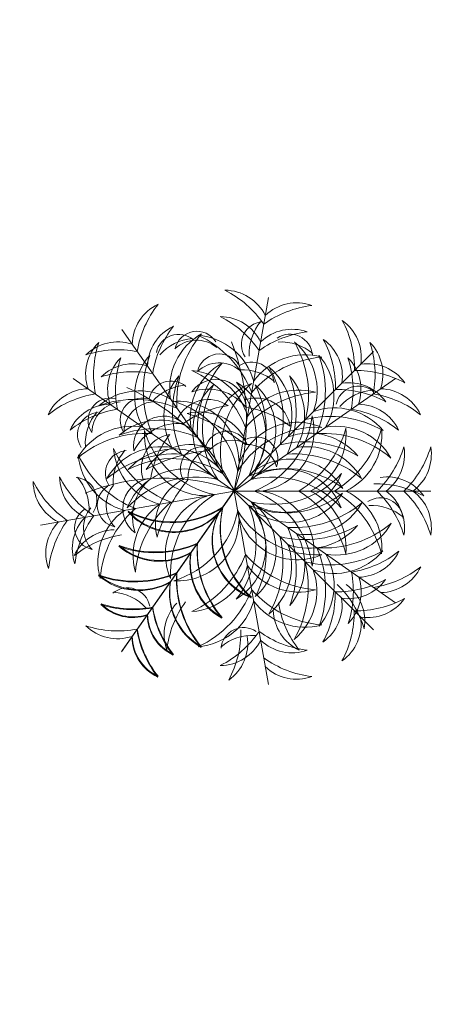
# Model space of a CAD drawing. Units: inches. Extents: x -48 to 50072, y 0 to 21068.
# Tile 23 of 75: x 341 to 369, y 289 to 353. Entities that reach past the tile are written whole.
import ezdxf

# ---------------------------------------------------------------- set-up
doc = ezdxf.new("R2010")
doc.units = ezdxf.units.IN
doc.header["$MEASUREMENT"] = 0
doc.layers.add('A-ANNO-DIMS', color=2, linetype='Continuous', lineweight=18)
doc.layers.add('L-PLNT', color=94, linetype='Continuous', lineweight=13)
doc.styles.get("Standard").update_dxf_attribs({"font": 'arial.ttf'})
doc.dimstyles.get("Standard").update_dxf_attribs({"dimtxt": 8, "dimasz": 0.18, "dimexe": 0.18, "dimexo": 0.0625, "dimgap": 0.09, "dimtad": 0, "dimtih": 1, "dimtoh": 1, "dimdec": 1, "dimzin": 0, "dimdsep": 46, "dimlunit": 4, "dimtxsty": 'Standard', "dimblk": 'ARCHTICK', "dimcen": 0.09, "dimadec": 0, "dimazin": 0, "dimtfac": 1, "dimtdec": 1, "dimtofl": 0, "dimtmove": 0, "dimatfit": 3, "dimldrblk": 'ARCHTICK', "dimfxl": 1, "dimtolj": 1, "dimtzin": 0, "dimarcsym": 0})

# ---------------------------------------------------------------- blocks, each defined once
blk = doc.blocks.new('A$C5D061C3B')
for p, q in [((3.377, 6.679), (3.377, 3.377)), ((1.483, 6.082), (3.377, 3.377)), ((5.259, 6.086), (3.365, 3.381)), ((1.03, 5.716), (3.365, 3.381)), ((5.712, 5.712), (3.377, 3.377)), ((0.125, 3.951), (3.377, 3.377)), ((6.629, 3.951), (3.377, 3.377)), ((0.66, 1.487), (3.365, 3.381)), ((1.483, 0.672), (3.377, 3.377)), ((6.07, 1.487), (3.365, 3.381)), ((3.951, 0.125), (3.377, 3.377)), ((6.082, 1.483), (3.377, 3.377))]:
    blk.add_line(p, q)
for centre, radius, start, end in [((2.763, 5.924), 0.762, 36.29, 99.6243), ((2.145, 5.032), 1.715, 44.0763, 73.3794), ((3.991, 5.924), 0.762, 80.3757, 143.71), ((4.61, 5.032), 1.715, 106.6206, 135.9237), ((2.419, 5.816), 0.762, 115.3757, 178.71), ((3.438, 5.44), 1.715, 141.6206, 170.9237), ((3.901, 5.939), 0.762, 125.3757, 188.71), ((4.969, 5.745), 1.715, 151.6206, 180.9237), ((3.305, 5.444), 1.715, 9.0763, 38.3794), ((4.323, 5.82), 0.762, 1.29, 64.6243), ((1.998, 5.617), 0.762, 125.3757, 188.71), ((3.066, 5.423), 1.715, 151.6206, 180.9237), ((2.678, 5.447), 0.762, 115.3757, 178.71), ((3.696, 5.07), 1.715, 141.6206, 170.9237), ((2.763, 5.474), 0.762, 36.29, 99.6243), ((2.145, 4.581), 1.715, 44.0763, 73.3794), ((3.991, 5.474), 0.762, 80.3757, 143.71), ((4.61, 4.581), 1.715, 106.6206, 135.9237), ((3.871, 5.832), 0.38, 94.742, 213.7475), ((4.447, 5.681), 0.826, 139.618, 183.2106), ((4.064, 5.451), 0.762, 1.29, 64.6243), ((3.046, 5.075), 1.715, 9.0763, 38.3794), ((4.744, 5.613), 0.762, 351.29, 54.6243), ((3.676, 5.419), 1.715, 359.0763, 28.3794), ((3.344, 5.089), 1.056, 119.6063, 189.7511), ((4.177, 4.869), 1.77, 139.9634, 183.6288), ((3.398, 5.094), 1.056, 350.2489, 60.3937), ((2.565, 4.873), 1.77, 356.3712, 40.0366), ((1.413, 5.111), 0.762, 71.29, 134.6243), ((2.317, 5.298), 0.762, 125.3757, 188.71), ((3.385, 5.104), 1.715, 151.6206, 180.9237), ((3.035, 5.062), 1.056, 129.6063, 199.7511), ((3.894, 4.989), 1.77, 149.9634, 193.6288), ((2.422, 4.799), 1.056, 25.2489, 95.3937), ((1.866, 4.14), 1.77, 31.3712, 75.0366), ((4.332, 4.799), 1.056, 84.6063, 154.7511), ((4.888, 4.14), 1.77, 104.9634, 148.6288), ((2.848, 4.985), 1.77, 346.3712, 30.0366), ((3.707, 5.058), 1.056, 340.2489, 50.3937), ((3.357, 5.1), 1.715, 359.0763, 28.3794), ((4.425, 5.294), 0.762, 351.29, 54.6243), ((1.419, 4.026), 1.715, 79.0763, 108.3794), ((1.991, 5.462), 0.38, 139.742, 258.7475), ((2.505, 5.763), 0.826, 184.618, 228.2106), ((1.13, 4.748), 0.762, 81.29, 144.6243), ((1.671, 4.742), 0.762, 71.29, 134.6243), ((3.688, 4.597), 1.056, 119.6063, 189.7511), ((4.522, 4.377), 1.77, 139.9634, 183.6288), ((2.221, 4.381), 1.77, 356.3712, 40.0366), ((3.054, 4.602), 1.056, 350.2489, 60.3937), ((5.071, 4.746), 0.762, 45.3757, 108.71), ((5.564, 4.807), 0.762, 80.3757, 143.71), ((6.182, 3.914), 1.715, 106.6206, 135.9237), ((5.613, 4.744), 0.762, 35.3757, 98.71), ((1.324, 3.68), 1.715, 89.0763, 118.3794), ((1.677, 3.657), 1.715, 79.0763, 108.3794), ((3.46, 4.637), 1.056, 129.6063, 199.7511), ((4.319, 4.565), 1.77, 149.9634, 193.6288), ((3.283, 4.633), 1.056, 340.2489, 50.3937), ((2.424, 4.56), 1.77, 346.3712, 30.0366), ((5.065, 3.661), 1.715, 71.6206, 100.9237), ((5.419, 3.676), 1.715, 61.6206, 90.9237), ((1.448, 4.43), 0.762, 81.29, 144.6243), ((2.422, 4.198), 1.056, 25.2489, 95.3937), ((1.866, 3.54), 1.77, 31.3712, 75.0366), ((3.868, 4.321), 1.029, 121.3654, 221.5741), ((4.556, 4.237), 1.557, 141.8122, 203.3335), ((4.035, 4.215), 1.029, 111.3654, 211.5741), ((2.707, 4.219), 1.029, 328.4259, 68.6346), ((2.044, 4.017), 1.557, 346.6665, 48.1878), ((4.698, 4.013), 1.557, 131.8122, 193.3335), ((4.332, 4.198), 1.056, 84.6063, 154.7511), ((4.888, 3.54), 1.77, 104.9634, 148.6288), ((2.187, 4.233), 1.557, 336.6665, 38.1878), ((2.875, 4.316), 1.029, 318.4259, 58.6346), ((5.294, 4.425), 0.762, 35.3757, 98.71), ((1.642, 3.362), 1.715, 89.0763, 118.3794), ((1.78, 3.994), 1.056, 60.2489, 130.3937), ((4.963, 3.998), 1.056, 49.6063, 119.7511), ((5.1, 3.357), 1.715, 61.6206, 90.9237), ((2.143, 4.564), 1.056, 164.6063, 234.7511), ((1.702, 3.136), 1.77, 66.3712, 110.0366), ((2.888, 4.998), 1.77, 184.9634, 228.6288), ((3.25, 4.435), 1.029, 156.3654, 256.5741), ((3.862, 4.761), 1.557, 176.8122, 238.3335), ((2.893, 4.761), 1.557, 301.6665, 3.1878), ((3.504, 4.435), 1.029, 283.4259, 23.6346), ((5.04, 3.14), 1.77, 69.9634, 113.6288), ((3.866, 4.998), 1.77, 311.3712, 355.0366), ((4.611, 4.564), 1.056, 305.2489, 15.3937), ((0.975, 4.424), 0.762, 160.3757, 223.71), ((1.962, 4.878), 1.715, 186.6206, 215.9237), ((1.12, 4.31), 0.38, 94.742, 213.7475), ((1.696, 4.159), 0.826, 139.618, 183.2106), ((1.685, 3.712), 1.056, 70.2489, 140.3937), ((2.734, 4.46), 1.056, 164.6063, 234.7511), ((3.48, 4.893), 1.77, 184.9634, 228.6288), ((2.358, 3.686), 1.029, 3.4259, 103.6346), ((1.93, 3.14), 1.557, 21.6665, 83.1878), ((4.397, 3.686), 1.029, 76.3654, 176.5741), ((4.824, 3.14), 1.557, 96.8122, 158.3335), ((3.275, 4.893), 1.77, 311.3712, 355.0366), ((4.02, 4.46), 1.056, 305.2489, 15.3937), ((5.058, 3.707), 1.056, 39.6063, 109.7511), ((4.793, 4.878), 1.715, 324.0763, 353.3794), ((5.779, 4.424), 0.762, 316.29, 19.6243), ((1.419, 4.346), 0.762, 160.3757, 223.71), ((2.405, 4.8), 1.715, 186.6206, 215.9237), ((1.757, 2.853), 1.77, 76.3712, 120.0366), ((2.124, 3.502), 1.056, 60.2489, 130.3937), ((4.618, 3.506), 1.056, 49.6063, 119.7511), ((4.985, 2.848), 1.77, 59.9634, 103.6288), ((4.349, 4.8), 1.715, 324.0763, 353.3794), ((5.335, 4.346), 0.762, 316.29, 19.6243), ((2.109, 3.287), 1.056, 70.2489, 140.3937), ((2.046, 2.644), 1.77, 66.3712, 110.0366), ((2.387, 3.752), 0.574, 99.9865, 199.4034), ((3.599, 3.314), 1.651, 142.5759, 170.8942), ((4.696, 2.648), 1.77, 69.9634, 113.6288), ((4.633, 3.283), 1.056, 39.6063, 109.7511), ((4.988, 5.812), 1.715, 279.0763, 308.3794), ((5.365, 4.794), 0.762, 271.29, 334.6243), ((2.182, 2.428), 1.77, 76.3712, 120.0366), ((4.56, 2.424), 1.77, 59.9634, 103.6288), ((1.588, 3.666), 0.38, 94.742, 213.7475), ((2.165, 3.515), 0.826, 139.618, 183.2106), ((2.365, 3.045), 1.029, 38.4259, 138.6346), ((2.84, 3.739), 0.372, 69.2257, 210.1279), ((3.109, 3.59), 0.515, 105.4398, 183.6694), ((4.377, 3.05), 1.029, 41.3654, 141.5741), ((0.762, 3.214), 0.762, 116.29, 179.6243), ((1.534, 2.451), 1.715, 124.0763, 153.3794), ((1.206, 3.136), 0.762, 116.29, 179.6243), ((1.062, 4.452), 0.826, 229.618, 273.2106), ((0.91, 3.875), 0.38, 184.742, 303.7475), ((2.426, 2.879), 1.029, 48.4259, 148.6346), ((2.328, 2.353), 1.557, 56.6665, 118.1878), ((4.414, 2.358), 1.557, 61.8122, 123.3335), ((4.316, 2.875), 1.029, 31.3654, 131.5741), ((5.549, 3.136), 0.762, 0.3757, 63.71), ((1.977, 2.373), 1.715, 124.0763, 153.3794), ((1.811, 2.684), 1.056, 105.2489, 175.3937), ((2.363, 2.022), 1.77, 111.3712, 155.0366), ((2.51, 2.191), 1.557, 66.6665, 128.1878), ((2.729, 4.702), 1.557, 221.8122, 283.3335), ((2.527, 4.039), 1.029, 201.3654, 301.5741), ((4.233, 2.187), 1.557, 51.8122, 113.3335), ((4.001, 4.702), 1.557, 256.6665, 318.1878), ((4.013, 4.698), 1.557, 256.6665, 318.1878), ((4.203, 4.039), 1.029, 238.4259, 338.6346), ((4.215, 4.035), 1.029, 238.4259, 338.6346), ((4.391, 2.022), 1.77, 24.9634, 68.6288), ((4.943, 2.684), 1.056, 4.6063, 74.7511), ((6.053, 3.533), 0.38, 146.2525, 265.258), ((4.777, 2.373), 1.715, 26.6206, 55.9237), ((6.629, 3.684), 0.826, 176.7894, 220.382), ((2.185, 0.015), 3.567, 70.4772, 111.6585), ((2.403, 2.58), 1.056, 105.2489, 175.3937), ((2.955, 1.917), 1.77, 111.3712, 155.0366), ((2.007, 3.071), 0.506, 93.8744, 233.9763), ((2.489, 2.932), 0.825, 128.7536, 199.097), ((2.903, 2.8), 0.855, 116.4477, 194.3672), ((4.744, 1.779), 2.789, 140.4007, 163.139), ((2.741, 3.253), 0.372, 114.2257, 255.1279), ((3.037, 3.338), 0.515, 150.4398, 228.6694), ((3.799, 1.917), 1.77, 24.9634, 68.6288), ((4.352, 2.58), 1.056, 4.6063, 74.7511), ((5.741, 1.774), 1.715, 61.6206, 90.9237), ((5.935, 2.842), 0.762, 35.3757, 98.71), ((1.447, 3.129), 0.376, 122.0577, 257.8533), ((1.751, 3.126), 0.529, 140.1845, 223.654), ((4.912, 0.157), 3.567, 115.4772, 156.6585), ((2.896, 2.427), 1.029, 83.4259, 183.6346), ((3.359, 1.911), 1.557, 101.6665, 163.1878), ((6.727, 2.189), 3.567, 160.4772, 201.6585), ((3.395, 1.911), 1.557, 16.8122, 78.3335), ((3.858, 2.427), 1.029, 356.3654, 96.5741), ((2.145, 3.693), 1.056, 209.6063, 279.7511), ((2.365, 4.526), 1.77, 229.9634, 273.6288), ((2.412, 2.943), 0.574, 144.9865, 244.4034), ((3.578, 3.49), 1.651, 187.5759, 215.8942), ((3.697, 2.369), 1.029, 128.4259, 228.6346), ((4.389, 2.332), 1.557, 146.6665, 208.1878), ((2.341, 2.332), 1.557, 331.8122, 33.3335), ((2.353, 2.328), 1.557, 331.8122, 33.3335), ((3.033, 2.369), 1.029, 311.3654, 51.5741), ((3.045, 2.365), 1.029, 311.3654, 51.5741), ((4.365, 4.526), 1.77, 266.3712, 310.0366), ((4.377, 4.522), 1.77, 266.3712, 310.0366), ((4.585, 3.693), 1.056, 260.2489, 330.3937), ((4.597, 3.688), 1.056, 260.2489, 330.3937), ((1.067, 2.749), 0.376, 122.0577, 257.8533), ((1.37, 2.745), 0.529, 140.1845, 223.654), ((2.328, 4.401), 1.557, 241.8122, 303.3335), ((2.365, 3.709), 1.029, 221.3654, 321.5741), ((1.911, 3.359), 1.557, 286.8122, 348.3335), ((2.427, 2.896), 1.029, 266.3654, 6.5741), ((4.035, 2.539), 1.029, 148.4259, 248.6346), ((4.698, 2.741), 1.557, 166.6665, 228.1878), ((4.435, 3.25), 1.029, 193.4259, 293.6346), ((4.761, 3.862), 1.557, 211.6665, 273.1878), ((1.873, 4.181), 1.77, 229.9634, 273.6288), ((1.653, 3.348), 1.056, 209.6063, 279.7511), ((3.45, 2.634), 0.855, 161.4477, 239.3672), ((3.003, 2.844), 0.372, 159.2257, 300.1279), ((3.152, 3.113), 0.515, 195.4398, 273.6694), ((5.474, 3.214), 2.789, 185.4007, 208.139), ((4.857, 4.181), 1.77, 266.3712, 310.0366), ((4.869, 4.177), 1.77, 266.3712, 310.0366), ((5.077, 3.348), 1.056, 260.2489, 330.3937), ((5.089, 3.344), 1.056, 260.2489, 330.3937), ((1.122, 2.441), 0.38, 139.742, 258.7475), ((1.636, 2.741), 0.826, 184.618, 228.2106), ((3.24, 2.128), 1.056, 150.2489, 220.3937), ((4.099, 2.051), 1.77, 156.3712, 200.0366), ((2.632, 2.051), 1.77, 339.9634, 23.6288), ((2.644, 2.046), 1.77, 339.9634, 23.6288), ((3.49, 2.128), 1.056, 319.6063, 29.7511), ((2.046, 4.111), 1.77, 249.9634, 293.6288), ((1.908, 2.317), 0.38, 139.742, 258.7475), ((2.422, 2.617), 0.826, 184.618, 228.2106), ((2.624, 2.192), 0.506, 138.8744, 278.9763), ((3.064, 2.435), 0.825, 173.7536, 244.097), ((4.522, 2.378), 1.77, 176.3712, 220.0366), ((3.942, 2.908), 0.855, 206.4477, 284.3672), ((4.963, 4.749), 2.789, 230.4007, 253.139), ((3.502, 2.124), 1.056, 319.6063, 29.7511), ((6.244, 3.948), 1.715, 234.0763, 263.3794), ((1.672, 3.7), 1.715, 231.6206, 260.9237), ((1.295, 2.682), 0.762, 205.3757, 268.71), ((2.124, 3.252), 1.056, 229.6063, 299.7511), ((3.607, 1.706), 1.77, 156.3712, 200.0366), ((3.688, 2.157), 1.056, 170.2489, 240.3937), ((3.124, 1.706), 1.77, 339.9634, 23.6288), ((3.136, 1.702), 1.77, 339.9634, 23.6288), ((5.79, 2.962), 0.762, 226.29, 289.6243), ((5.058, 3.7), 1.715, 279.0763, 308.3794), ((5.07, 3.696), 1.715, 279.0763, 308.3794), ((5.435, 2.682), 0.762, 271.29, 334.6243), ((5.447, 2.678), 0.762, 271.29, 334.6243), ((2.748, 1.784), 1.056, 150.2489, 220.3937), ((3.428, 3.603), 1.651, 232.5759, 260.8942), ((2.99, 2.391), 0.574, 189.9865, 289.4034), ((1.917, 2.955), 1.77, 294.9634, 338.6288), ((4.893, 3.48), 1.77, 221.3712, 265.0366), ((3.982, 1.784), 1.056, 319.6063, 29.7511), ((3.994, 1.78), 1.056, 319.6063, 29.7511), ((0.926, 2.424), 0.762, 205.3757, 268.71), ((1.303, 3.442), 1.715, 231.6206, 260.9237), ((1.702, 3.619), 1.77, 249.9634, 293.6288), ((3.086, 1.681), 1.715, 169.0763, 198.3794), ((2.405, 2.049), 0.529, 185.1845, 268.654), ((4.177, 1.886), 1.77, 176.3712, 220.0366), ((2.58, 2.403), 1.056, 274.6063, 344.7511), ((4.46, 2.734), 1.056, 215.2489, 285.3937), ((3.645, 1.681), 1.715, 341.6206, 10.9237), ((3.657, 1.677), 1.715, 341.6206, 10.9237), ((5.427, 3.442), 1.715, 279.0763, 308.3794), ((5.44, 3.438), 1.715, 279.0763, 308.3794), ((5.804, 2.424), 0.762, 271.29, 334.6243), ((5.816, 2.419), 0.762, 271.29, 334.6243), ((1.78, 2.76), 1.056, 229.6063, 299.7511), ((2, 1.676), 0.762, 161.29, 224.6243), ((2.188, 1.837), 0.376, 167.0577, 302.8533), ((3.344, 1.665), 1.056, 170.2489, 240.3937), ((3.81, 2.493), 0.825, 218.7536, 289.097), ((3.671, 2.011), 0.506, 183.8744, 323.9763), ((5.385, 1.584), 0.38, 101.2525, 220.258), ((5.899, 1.283), 0.826, 131.7894, 175.382), ((4.73, 1.676), 0.762, 315.3757, 18.71), ((4.742, 1.671), 0.762, 315.3757, 18.71), ((1.631, 1.417), 0.762, 161.29, 224.6243), ((2.717, 1.423), 1.715, 169.0763, 198.3794), ((2.022, 2.363), 1.77, 294.9634, 338.6288), ((4.998, 2.888), 1.77, 221.3712, 265.0366), ((4.014, 1.423), 1.715, 341.6206, 10.9237), ((5.099, 1.417), 0.762, 315.3757, 18.71), ((3.227, 2.169), 0.826, 229.618, 273.2106), ((3.076, 1.593), 0.38, 184.742, 303.7475), ((2.684, 1.811), 1.056, 274.6063, 344.7511), ((4.564, 2.143), 1.056, 215.2489, 285.3937), ((1.671, 2.012), 0.762, 225.3757, 288.71), ((1.677, 3.098), 1.715, 251.6206, 280.9237), ((2.188, 1.299), 0.376, 167.0577, 302.8533), ((2.405, 1.511), 0.529, 185.1845, 268.654), ((3.696, 1.684), 1.715, 189.0763, 218.3794), ((3.616, 1.755), 0.529, 230.1845, 313.654), ((3.613, 1.452), 0.376, 212.0577, 347.8533), ((4.79, 1.377), 0.762, 181.29, 244.6243), ((5.808, 1.754), 1.715, 189.0763, 218.3794), ((2.678, 1.307), 0.762, 181.29, 244.6243), ((1.419, 2.729), 1.715, 251.6206, 280.9237), ((1.413, 1.643), 0.762, 225.3757, 288.71), ((3.438, 1.315), 1.715, 189.0763, 218.3794), ((2.583, 1.701), 0.826, 229.618, 273.2106), ((2.432, 1.124), 0.38, 184.742, 303.7475), ((2.373, 1.977), 1.715, 296.6206, 325.9237), ((3.528, 0.69), 0.38, 56.2525, 175.258), ((4.8, 2.405), 1.715, 234.0763, 263.3794), ((2.419, 0.938), 0.762, 181.29, 244.6243), ((3.136, 1.206), 0.762, 270.3757, 333.71), ((3.68, 0.113), 0.826, 86.7894, 130.382), ((3.997, 1.374), 0.529, 230.1845, 313.654), ((3.994, 1.071), 0.376, 212.0577, 347.8533), ((4.346, 1.419), 0.762, 226.29, 289.6243), ((2.451, 1.534), 1.715, 296.6206, 325.9237), ((4.878, 1.962), 1.715, 234.0763, 263.3794), ((3.214, 0.762), 0.762, 270.3757, 333.71), ((4.424, 0.975), 0.762, 226.29, 289.6243)]:
    blk.add_arc(centre, radius, start, end)
blk = doc.blocks.new('_ArchTick')
at = {"color": 0, "linetype": 'ByBlock', "const_width": 0.15}
blk.add_lwpolyline([(-0.5, -0.5), (0.5, 0.5)], dxfattribs=at)
blk = doc.blocks.new('*D118')
at = {"layer": 'A-ANNO-DIMS', "color": 0, "lineweight": -2, "transparency": 16777216}
for p, q in [((297.017, 488.712), (297.017, 165.945)), ((463.517, 488.712), (463.517, 165.945)), ((297.017, 166.125), (367.026, 166.125)), ((463.517, 166.125), (393.509, 166.125))]:
    blk.add_line(p, q, dxfattribs=at)
at = {"layer": 'Defpoints', "color": 0, "transparency": 16777216}
for p in [(297.017, 488.775), (463.517, 488.775), (463.517, 166.125)]:
    blk.add_point(p, dxfattribs=at)
at = {"layer": 'A-ANNO-DIMS', "color": 0, "lineweight": -2, "transparency": 16777216, "xscale": 0.18, "yscale": 0.18, "zscale": 0.18, "rotation": 180}
blk.add_blockref('_ArchTick', (297.017, 166.125), dxfattribs=at)
at = {"layer": 'A-ANNO-DIMS', "color": 0, "lineweight": -2, "transparency": 16777216, "xscale": 0.18, "yscale": 0.18, "zscale": 0.18}
blk.add_blockref('_ArchTick', (463.517, 166.125), dxfattribs=at)
at = {"layer": 'A-ANNO-DIMS', "color": 0, "transparency": 16777216, "insert": (380.267, 166.125), "char_height": 8, "attachment_point": 5}
blk.add_mtext('\\A1;166.5', dxfattribs=at)

msp = doc.modelspace()

# ---------------------------------------------------------------- block references
at = {"layer": 'L-PLNT', "xscale": 3.862191520948588, "yscale": 3.862191520948588, "zscale": 3.862191520948588, "rotation": 270}
msp.add_blockref('A$C5D061C3B', (342.069, 335.125), dxfattribs=at)

# ---------------------------------------------------------------- dimensions: what is measured, and where the dimension line sits
at = {"layer": 'A-ANNO-DIMS'}
dim = msp.add_linear_dim(base=(463.517, 166.125), p1=(297.017, 488.775), p2=(463.517, 488.775), dimstyle='Standard', override={"dimdec": 1, "dimlfac": 1, "dimrnd": 0, "dimzin": 0, "dimdsep": 46, "dimlunit": 2}, dxfattribs=at)
dim.commit()
dim.dimension.update_dxf_attribs({"geometry": '*D118', "text_midpoint": (380.267, 166.125)})

doc.saveas('drawing.dxf')
